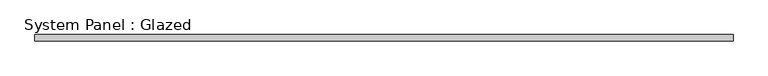
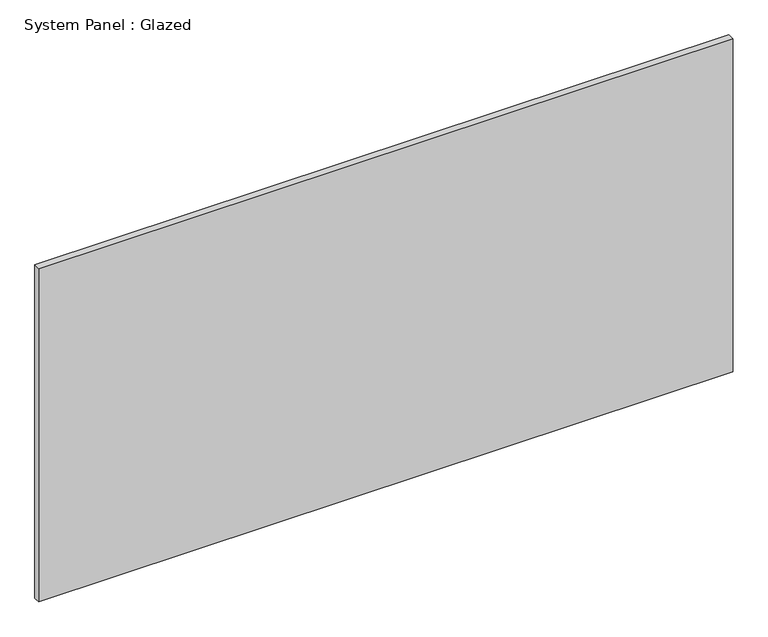
"""IFC4 building model written with IfcOpenShell, lengths in millimetres: plate geometry, System Panel : Glazed."""

from ifc_helpers import new_model, si_unit, origin, origin_with_axes, place, context, project, spatial, polyline, outline, extrude, source, transform, mapped, element, save


def system_panel_glazed_7fb1fc2b(model_context):
    return source(origin(), model_context, "Body", "SweptSolid", [
        extrude(outline(polyline([(1408.2170105, 19.05), (-1408.2170105, 19.05), (-1408.2170105, 44.45), (1408.2170105, 44.45), (1408.2170105, 19.05)])), origin_with_axes(), (0.0, 0.0, 1.0), 1428.75),
    ])


if __name__ == "__main__":
    model = new_model("IFC4")
    model_context = context("Model", 3, world=origin())
    ifc_project = project(units=[si_unit("LENGTHUNIT", "METRE", prefix="MILLI")], contexts=[model_context])
    site = spatial("IfcSite", under=ifc_project)
    building = spatial("IfcBuilding", under=site)
    placement = place(None, origin())
    system_panel_glazed_shape = system_panel_glazed_7fb1fc2b(model_context)
    element("IfcPlate", 1, ObjectType="System Panel : Glazed", at=placement, inside=building, context=model_context, shape_type="MappedRepresentation", body=[
        mapped(system_panel_glazed_shape, transform((0.0, 0.0, 0.0), x_axis=(1.0, 0.0, 0.0), y_axis=(0.0, 1.0, 0.0), z_axis=(0.0, 0.0, 1.0))),
    ])
    save(model, "model.ifc")

# Revit data of these elements
# Type "System Panel : Glazed"
#   Construction Type Id = "GSP4R"
#   Analytic Construction = "1/8 in Pilkington single glazing"
#   Visual Light Transmittance = 0.9
#   Solar Heat Gain Coefficient = 0.86
#   Heat Transfer Coefficient (U) = 1.18115 BTU/(h·ft²·°F)
#   Define Thermal Properties by = 1
# Element 1 (IfcPlate, "System Panel : Glazed")
#   Materials on its faces: "Glass"
# Materials
#   "Glass": class "Glass", colour RGB 0 128 192, transparency 0.75, Description = "Soda Lime Glass", Cost = 0
